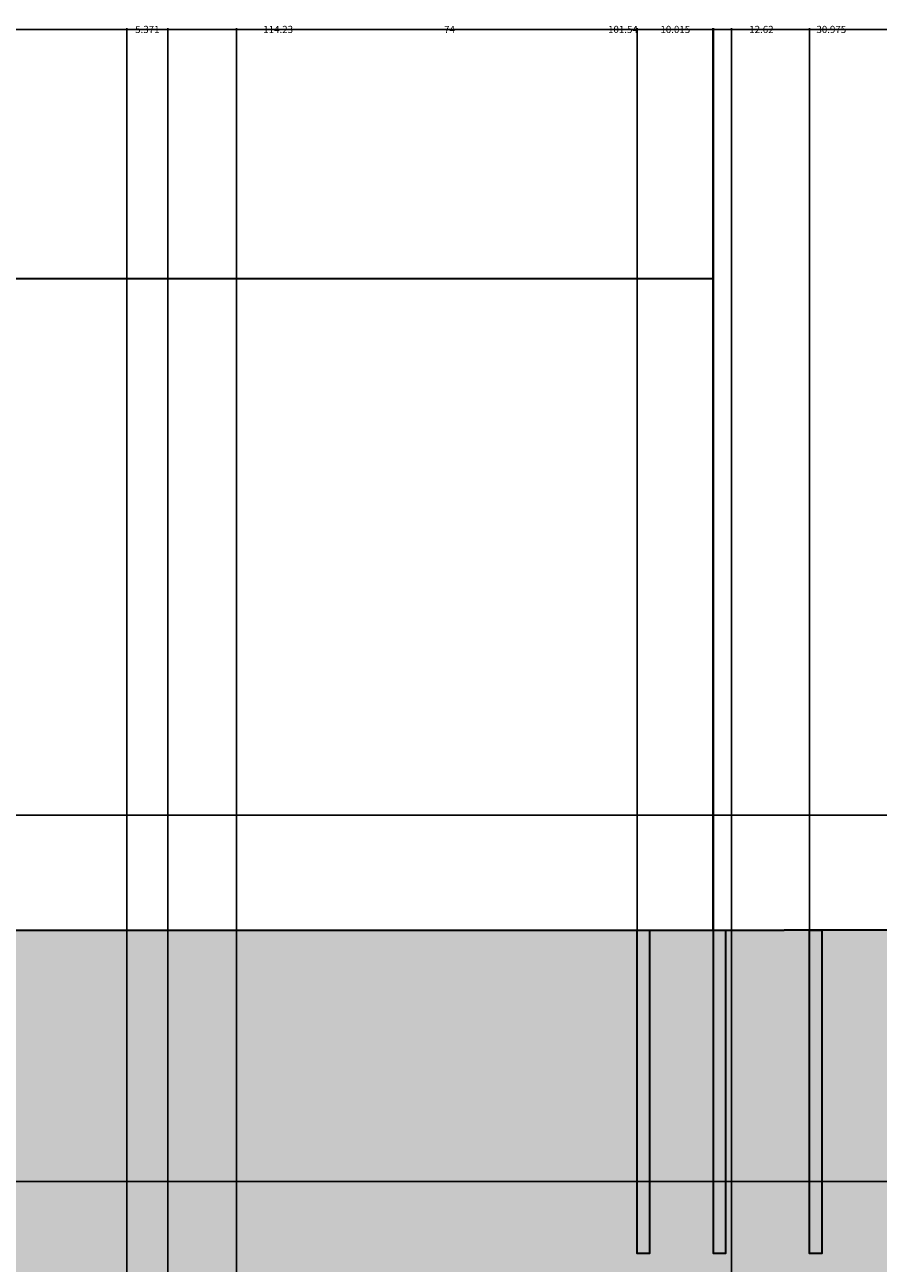
# Model space of a CAD drawing. Units: inches. Extents: x -5 to 714, y 84 to 644.
# Tile 10 of 20: x 108 to 220, y 481 to 644. Entities that reach past the tile are written whole.
import ezdxf

# ---------------------------------------------------------------- set-up
doc = ezdxf.new("R2010")
doc.units = ezdxf.units.IN
doc.header["$MEASUREMENT"] = 0
for name, color, linetype, lineweight in [('A-ANNO-DIMS', 2, 'Continuous', 18), ('A-ELEV', 7, 'Continuous', 35), ('A-ELEV-PATT', 8, 'Continuous', 13)]:
    doc.layers.add(name, color=color, linetype=linetype, lineweight=lineweight)
doc.styles.get("Standard").update_dxf_attribs({"font": 'arial.ttf'})
doc.dimstyles.get("Standard").update_dxf_attribs({"dimtxt": 0.9375, "dimasz": 0.18, "dimexe": 0.18, "dimexo": 0.0625, "dimgap": 0.09, "dimtad": 0, "dimtih": 1, "dimtoh": 1, "dimdec": 4, "dimzin": 0, "dimdsep": 46, "dimlunit": 4, "dimtxsty": 'Standard', "dimcen": 0.09, "dimadec": 0, "dimazin": 0, "dimtfac": 1, "dimtdec": 4, "dimtofl": 0, "dimtmove": 0, "dimatfit": 3, "dimfxl": 1, "dimtolj": 1, "dimtzin": 0, "dimarcsym": 0})

# ---------------------------------------------------------------- blocks, each defined once
blk = doc.blocks.new('*D10')
at = {"layer": 'A-ANNO-DIMS', "color": 0, "lineweight": -2, "transparency": 16777216}
for p, q in [((84.1, 610.79), (84.1, 643.61)), ((84.28, 643.43), (139.22, 643.43)), ((198.15, 643.43), (143.21, 643.43)), ((198.33, 610.79), (198.33, 643.61))]:
    blk.add_line(p, q, dxfattribs=at)
at = {"layer": 'A-ANNO-DIMS', "color": 0, "transparency": 16777216}
for points in [[(84.28, 643.46), (84.28, 643.4), (84.1, 643.43)], [(198.15, 643.46), (198.15, 643.4), (198.33, 643.43)]]:
    blk.add_solid(points, dxfattribs=at)
at = {"layer": 'Defpoints', "color": 0, "transparency": 16777216}
for p in [(198.33, 643.43), (84.1, 610.73), (198.33, 610.73)]:
    blk.add_point(p, dxfattribs=at)
at = {"layer": 'A-ANNO-DIMS', "color": 0, "transparency": 16777216, "insert": (141.22, 643.43), "char_height": 0.938, "attachment_point": 5}
blk.add_mtext('\\A1;114.23', dxfattribs=at)
blk = doc.blocks.new('*D11')
at = {"layer": 'A-ANNO-DIMS', "color": 0, "lineweight": -2, "transparency": 16777216}
for p, q in [((198.38, 525.26), (198.38, 643.61)), ((198.56, 643.43), (211.83, 643.43)), ((229.18, 643.43), (215.91, 643.43)), ((229.36, 525.26), (229.36, 643.61))]:
    blk.add_line(p, q, dxfattribs=at)
at = {"layer": 'A-ANNO-DIMS', "color": 0, "transparency": 16777216}
for points in [[(198.56, 643.46), (198.56, 643.4), (198.38, 643.43)], [(229.18, 643.46), (229.18, 643.4), (229.36, 643.43)]]:
    blk.add_solid(points, dxfattribs=at)
at = {"layer": 'Defpoints', "color": 0, "transparency": 16777216}
for p in [(229.36, 643.43), (198.38, 525.19), (229.36, 525.19)]:
    blk.add_point(p, dxfattribs=at)
at = {"layer": 'A-ANNO-DIMS', "color": 0, "transparency": 16777216, "insert": (213.87, 643.43), "char_height": 0.938, "attachment_point": 5}
blk.add_mtext('\\A1;30.975', dxfattribs=at)
blk = doc.blocks.new('*D16')
at = {"layer": 'A-ANNO-DIMS', "color": 0, "lineweight": -2, "transparency": 16777216}
for p, q in [((364.22, 540.29), (-2.74, 540.29)), ((-2.56, 540.11), (-2.56, 510.8)), ((-2.56, 480.35), (-2.56, 509.66)), ((364.22, 480.17), (-2.74, 480.17))]:
    blk.add_line(p, q, dxfattribs=at)
at = {"layer": 'A-ANNO-DIMS', "color": 0, "transparency": 16777216}
for points in [[(-2.59, 540.11), (-2.53, 540.11), (-2.56, 540.29)], [(-2.59, 480.35), (-2.53, 480.35), (-2.56, 480.17)]]:
    blk.add_solid(points, dxfattribs=at)
at = {"layer": 'Defpoints', "color": 0, "transparency": 16777216}
for p in [(-2.56, 540.29), (364.28, 540.29), (364.28, 480.17)]:
    blk.add_point(p, dxfattribs=at)
at = {"layer": 'A-ANNO-DIMS', "color": 0, "transparency": 16777216, "insert": (-2.56, 510.23), "char_height": 0.938, "attachment_point": 5}
blk.add_mtext('\\A1;60.11', dxfattribs=at)
blk = doc.blocks.new('*D17')
at = {"layer": 'A-ANNO-DIMS', "color": 0, "lineweight": -2, "transparency": 16777216}
for p, q in [((338.04, 525.19), (-2.74, 525.19)), ((-2.56, 525.01), (-2.56, 509.25)), ((-2.56, 492.35), (-2.56, 508.11)), ((338.04, 492.17), (-2.74, 492.17))]:
    blk.add_line(p, q, dxfattribs=at)
at = {"layer": 'A-ANNO-DIMS', "color": 0, "transparency": 16777216}
for points in [[(-2.59, 525.01), (-2.53, 525.01), (-2.56, 525.19)], [(-2.59, 492.35), (-2.53, 492.35), (-2.56, 492.17)]]:
    blk.add_solid(points, dxfattribs=at)
at = {"layer": 'Defpoints', "color": 0, "transparency": 16777216}
for p in [(-2.56, 525.19), (338.11, 525.19), (338.11, 492.17)]:
    blk.add_point(p, dxfattribs=at)
at = {"layer": 'A-ANNO-DIMS', "color": 0, "transparency": 16777216, "insert": (-2.56, 508.68), "char_height": 0.938, "attachment_point": 5}
blk.add_mtext('\\A1;33.03', dxfattribs=at)
blk = doc.blocks.new('*D21')
at = {"layer": 'A-ANNO-DIMS', "color": 0, "lineweight": -2, "transparency": 16777216}
for p, q in [((188.37, 482.78), (188.37, 643.61)), ((188.55, 643.43), (191.38, 643.43)), ((198.2, 643.43), (195.37, 643.43)), ((198.38, 482.78), (198.38, 643.61))]:
    blk.add_line(p, q, dxfattribs=at)
at = {"layer": 'A-ANNO-DIMS', "color": 0, "transparency": 16777216}
for points in [[(188.55, 643.46), (188.55, 643.4), (188.37, 643.43)], [(198.2, 643.46), (198.2, 643.4), (198.38, 643.43)]]:
    blk.add_solid(points, dxfattribs=at)
at = {"layer": 'Defpoints', "color": 0, "transparency": 16777216}
for p in [(198.38, 643.43), (188.37, 482.72), (198.38, 482.72)]:
    blk.add_point(p, dxfattribs=at)
at = {"layer": 'A-ANNO-DIMS', "color": 0, "transparency": 16777216, "insert": (193.38, 643.43), "char_height": 0.938, "attachment_point": 5}
blk.add_mtext('\\A1;10.015', dxfattribs=at)
blk = doc.blocks.new('*D22')
at = {"layer": 'A-ANNO-DIMS', "color": 0, "lineweight": -2, "transparency": 16777216}
for p, q in [((198.38, 482.78), (198.38, 643.61)), ((198.56, 643.43), (203.07, 643.43)), ((210.82, 643.43), (206.32, 643.43)), ((211, 482.78), (211, 643.61))]:
    blk.add_line(p, q, dxfattribs=at)
at = {"layer": 'A-ANNO-DIMS', "color": 0, "transparency": 16777216}
for points in [[(198.56, 643.46), (198.56, 643.4), (198.38, 643.43)], [(210.82, 643.46), (210.82, 643.4), (211, 643.43)]]:
    blk.add_solid(points, dxfattribs=at)
at = {"layer": 'Defpoints', "color": 0, "transparency": 16777216}
for p in [(211, 643.43), (198.38, 482.72), (211, 482.72)]:
    blk.add_point(p, dxfattribs=at)
at = {"layer": 'A-ANNO-DIMS', "color": 0, "transparency": 16777216, "insert": (204.69, 643.43), "char_height": 0.938, "attachment_point": 5}
blk.add_mtext('\\A1;12.62', dxfattribs=at)
blk = doc.blocks.new('*D23')
at = {"layer": 'A-ANNO-DIMS', "color": 0, "lineweight": -2, "transparency": 16777216}
for p, q in [((229.3, 525.19), (-2.74, 525.19)), ((-2.56, 525.01), (-2.56, 503.25)), ((-2.56, 480.35), (-2.56, 502.11)), ((229.3, 480.17), (-2.74, 480.17))]:
    blk.add_line(p, q, dxfattribs=at)
at = {"layer": 'A-ANNO-DIMS', "color": 0, "transparency": 16777216}
for points in [[(-2.59, 525.01), (-2.53, 525.01), (-2.56, 525.19)], [(-2.59, 480.35), (-2.53, 480.35), (-2.56, 480.17)]]:
    blk.add_solid(points, dxfattribs=at)
at = {"layer": 'Defpoints', "color": 0, "transparency": 16777216}
for p in [(-2.56, 525.19), (229.36, 525.19), (229.36, 480.17)]:
    blk.add_point(p, dxfattribs=at)
at = {"layer": 'A-ANNO-DIMS', "color": 0, "transparency": 16777216, "insert": (-2.56, 502.68), "char_height": 0.938, "attachment_point": 5}
blk.add_mtext('\\A1;45.02', dxfattribs=at)
blk = doc.blocks.new('*D24')
at = {"layer": 'A-ANNO-DIMS', "color": 0, "lineweight": -2, "transparency": 16777216}
for p, q in [((126.73, 480.23), (126.73, 643.61)), ((126.91, 643.43), (295.25, 643.43)), ((466.92, 643.43), (298.58, 643.43)), ((467.1, 480.23), (467.1, 643.61))]:
    blk.add_line(p, q, dxfattribs=at)
at = {"layer": 'A-ANNO-DIMS', "color": 0, "transparency": 16777216}
for points in [[(126.91, 643.46), (126.91, 643.4), (126.73, 643.43)], [(466.92, 643.46), (466.92, 643.4), (467.1, 643.43)]]:
    blk.add_solid(points, dxfattribs=at)
at = {"layer": 'Defpoints', "color": 0, "transparency": 16777216}
for p in [(467.1, 643.43), (126.73, 480.17), (467.1, 480.17)]:
    blk.add_point(p, dxfattribs=at)
at = {"layer": 'A-ANNO-DIMS', "color": 0, "transparency": 16777216, "insert": (296.91, 643.43), "char_height": 0.938, "attachment_point": 5}
blk.add_mtext('\\A1;340.4', dxfattribs=at)
blk = doc.blocks.new('*D31')
at = {"layer": 'A-ANNO-DIMS', "color": 0, "lineweight": -2, "transparency": 16777216}
for p, q in [((135.73, 345.26), (135.73, 643.61)), ((135.91, 643.43), (184.51, 643.43)), ((237.09, 643.43), (188.49, 643.43)), ((237.27, 345.26), (237.27, 643.61))]:
    blk.add_line(p, q, dxfattribs=at)
at = {"layer": 'A-ANNO-DIMS', "color": 0, "transparency": 16777216}
for points in [[(135.91, 643.46), (135.91, 643.4), (135.73, 643.43)], [(237.09, 643.46), (237.09, 643.4), (237.27, 643.43)]]:
    blk.add_solid(points, dxfattribs=at)
at = {"layer": 'Defpoints', "color": 0, "transparency": 16777216}
for p in [(237.27, 643.43), (135.73, 345.19), (237.27, 345.19)]:
    blk.add_point(p, dxfattribs=at)
at = {"layer": 'A-ANNO-DIMS', "color": 0, "transparency": 16777216, "insert": (186.5, 643.43), "char_height": 0.938, "attachment_point": 5}
blk.add_mtext('\\A1;101.54', dxfattribs=at)
blk = doc.blocks.new('*D47')
at = {"layer": 'A-ANNO-DIMS', "color": 0, "lineweight": -2, "transparency": 16777216}
for p, q in [((75.5, 336.27), (75.5, 643.61)), ((75.68, 643.43), (96.74, 643.43)), ((121.18, 643.43), (100.13, 643.43)), ((121.36, 336.27), (121.36, 643.61))]:
    blk.add_line(p, q, dxfattribs=at)
at = {"layer": 'A-ANNO-DIMS', "color": 0, "transparency": 16777216}
for points in [[(75.68, 643.46), (75.68, 643.4), (75.5, 643.43)], [(121.18, 643.46), (121.18, 643.4), (121.36, 643.43)]]:
    blk.add_solid(points, dxfattribs=at)
at = {"layer": 'Defpoints', "color": 0, "transparency": 16777216}
for p in [(121.36, 643.43), (75.5, 336.21), (121.36, 336.21)]:
    blk.add_point(p, dxfattribs=at)
at = {"layer": 'A-ANNO-DIMS', "color": 0, "transparency": 16777216, "insert": (98.43, 643.43), "char_height": 0.938, "attachment_point": 5}
blk.add_mtext('\\A1;45.85', dxfattribs=at)
blk = doc.blocks.new('*D48')
at = {"layer": 'A-ANNO-DIMS', "color": 0, "lineweight": -2, "transparency": 16777216}
for p, q in [((121.36, 336.27), (121.36, 643.61)), ((121.54, 643.43), (122.46, 643.43)), ((126.55, 643.43), (125.63, 643.43)), ((126.73, 345.26), (126.73, 643.61))]:
    blk.add_line(p, q, dxfattribs=at)
at = {"layer": 'A-ANNO-DIMS', "color": 0, "transparency": 16777216}
for points in [[(121.54, 643.46), (121.54, 643.4), (121.36, 643.43)], [(126.55, 643.46), (126.55, 643.4), (126.73, 643.43)]]:
    blk.add_solid(points, dxfattribs=at)
at = {"layer": 'Defpoints', "color": 0, "transparency": 16777216}
for p in [(126.73, 643.43), (126.73, 345.19), (121.36, 336.21)]:
    blk.add_point(p, dxfattribs=at)
at = {"layer": 'A-ANNO-DIMS', "color": 0, "transparency": 16777216, "insert": (124.04, 643.43), "char_height": 0.938, "attachment_point": 5}
blk.add_mtext('\\A1;5.371', dxfattribs=at)
blk = doc.blocks.new('*D49')
at = {"layer": 'A-ANNO-DIMS', "color": 0, "lineweight": -2, "transparency": 16777216}
for p, q in [((126.73, 302), (126.73, 643.61)), ((126.91, 643.43), (162.98, 643.43)), ((200.56, 643.43), (164.49, 643.43)), ((200.74, 302), (200.74, 643.61))]:
    blk.add_line(p, q, dxfattribs=at)
at = {"layer": 'A-ANNO-DIMS', "color": 0, "transparency": 16777216}
for points in [[(126.91, 643.46), (126.91, 643.4), (126.73, 643.43)], [(200.56, 643.46), (200.56, 643.4), (200.74, 643.43)]]:
    blk.add_solid(points, dxfattribs=at)
at = {"layer": 'Defpoints', "color": 0, "transparency": 16777216}
for p in [(200.74, 643.43), (126.73, 301.94), (200.74, 301.94)]:
    blk.add_point(p, dxfattribs=at)
at = {"layer": 'A-ANNO-DIMS', "color": 0, "transparency": 16777216, "insert": (163.73, 643.43), "char_height": 0.938, "attachment_point": 5}
blk.add_mtext('\\A1;74', dxfattribs=at)
blk = doc.blocks.new('*D51')
at = {"layer": 'A-ANNO-DIMS', "color": 0, "lineweight": -2, "transparency": 16777216}
for p, q in [((200.74, 201.26), (200.74, 643.61)), ((200.92, 643.43), (223.39, 643.43)), ((249.24, 643.43), (226.77, 643.43)), ((249.42, 201.26), (249.42, 643.61))]:
    blk.add_line(p, q, dxfattribs=at)
at = {"layer": 'A-ANNO-DIMS', "color": 0, "transparency": 16777216}
for points in [[(200.92, 643.46), (200.92, 643.4), (200.74, 643.43)], [(249.24, 643.46), (249.24, 643.4), (249.42, 643.43)]]:
    blk.add_solid(points, dxfattribs=at)
at = {"layer": 'Defpoints', "color": 0, "transparency": 16777216}
for p in [(249.42, 643.43), (200.74, 201.19), (249.42, 201.19)]:
    blk.add_point(p, dxfattribs=at)
at = {"layer": 'A-ANNO-DIMS', "color": 0, "transparency": 16777216, "insert": (225.08, 643.43), "char_height": 0.938, "attachment_point": 5}
blk.add_mtext('\\A1;48.68', dxfattribs=at)

msp = doc.modelspace()

# ---------------------------------------------------------------- hatches: boundary and pattern name
at = {"layer": 'A-ELEV-PATT', "transparency": 33554687}
h = msp.add_hatch(color=256, dxfattribs=at)
h.dxf.hatch_style = 1
h.paths.add_polyline_path([(188.3677, 525.1928), (67.9893, 525.1928), (67.9893, 489.1928), (67.9893, 345.1928), (126.7303, 345.1928), (126.7303, 480.1709), (229.3575, 480.1709), (229.3575, 525.1928), (212.6043, 525.1928), (212.6043, 482.7164), (211.0019, 482.7164), (211.0019, 525.1928), (207.6919, 525.1928), (199.9852, 525.1928), (199.9852, 482.7164), (198.3828, 482.7164), (198.3828, 525.1928), (189.9701, 525.1928), (189.9701, 482.7164), (188.3677, 482.7164)])
h.paths.add_polyline_path([(121.3589, 336.2066), (75.5048, 336.2066), (75.5048, 319.345), (121.3589, 319.345)])
h.paths.add_polyline_path([(121.3589, 319.345), (75.5048, 319.345), (75.5048, 302.3045), (121.3589, 302.3045)])
h.paths.add_polyline_path([(121.3589, 302.3045), (75.5048, 302.3045), (75.5048, 282.8561), (121.3589, 282.8561)])
h.paths.add_polyline_path([(121.3589, 282.8561), (75.5048, 282.8561), (75.5048, 261.5556), (121.3589, 261.5556)])
h.paths.add_polyline_path([(121.3589, 261.5556), (75.5048, 261.5556), (75.5048, 243.7009), (121.3589, 243.7009)])
h.paths.add_polyline_path([(121.3589, 243.7009), (75.5048, 243.7009), (75.5048, 223.5117), (121.3589, 223.5117)])
h.paths.add_polyline_path([(121.3589, 223.5117), (75.5048, 223.5117), (75.5048, 212.5836), (121.3589, 212.5836)])
h.paths.add_polyline_path([(121.3589, 212.5836), (75.5048, 212.5836), (75.5048, 201.1928), (121.3589, 201.1928)])
h.paths.add_polyline_path([(179.9335, 201.1928), (30.1395, 201.1928), (30.1395, 198.7054), (179.9335, 198.7054)])
h.paths.add_polyline_path([(187.6349, 201.1928), (179.9335, 201.1928), (179.9335, 198.7054), (179.9335, 141.1928), (269.2446, 141.1928), (269.2446, 201.1928), (263.4349, 201.1928), (263.4349, 152.1176), (187.6349, 152.1176)])
h.paths.add_polyline_path([(269.2446, 277.0513), (269.2446, 287.501), (269.2446, 306.6286), (578.0915, 306.6286), (578.0915, 201.1928), (593.428, 201.1928), (593.428, 315.0968), (584.4202, 315.0968), (259.0665, 315.0968), (259.0665, 201.1928), (263.4349, 201.1928), (269.2446, 201.1928)])
h = msp.add_hatch(color=256, dxfattribs=at)
h.dxf.hatch_style = 1
h.paths.add_polyline_path([(189.9701, 525.1928), (188.3677, 525.1928), (188.3677, 482.7164), (189.9701, 482.7164)])
h.paths.add_polyline_path([(199.9852, 525.1928), (198.3828, 525.1928), (198.3828, 482.7164), (199.9852, 482.7164)])
h.paths.add_polyline_path([(212.6043, 525.1928), (211.0019, 525.1928), (211.0019, 482.7164), (212.6043, 482.7164)])

# ---------------------------------------------------------------- linework, layer by layer
at = {"layer": 'A-ELEV'}
for p, q in [((79.1019, 610.7276), (198.3291, 610.7276)), ((198.3291, 610.7276), (198.3291, 525.1928)), ((67.9893, 525.1928), (207.6919, 525.1928)), ((229.3575, 525.1928), (207.6919, 525.1928))]:
    msp.add_line(p, q, dxfattribs=at)
for points in [[(188.3677, 525.1928), (189.9701, 525.1928), (189.9701, 482.7164), (188.3677, 482.7164)], [(198.3828, 525.1928), (199.9852, 525.1928), (199.9852, 482.7164), (198.3828, 482.7164)], [(211.0019, 525.1928), (212.6043, 525.1928), (212.6043, 482.7164), (211.0019, 482.7164)]]:
    msp.add_lwpolyline(points, close=True, dxfattribs=at)

# ---------------------------------------------------------------- dimensions: what is measured, and where the dimension line sits
at = {"layer": 'A-ANNO-DIMS'}
for base, p1, p2, override, picture, middle in [((121.3589, 643.4276), (75.5048, 336.2066), (121.3589, 336.2066), {"dimdec": 2, "dimlfac": 1, "dimrnd": 0, "dimzin": 0, "dimdsep": 46, "dimlunit": 2}, '*D47', (98.4319, 643.4276)), ((198.3291, 643.4276), (84.1027, 610.7276), (198.3291, 610.7276), {"dimdec": 2, "dimlfac": 1, "dimrnd": 0, "dimzin": 0, "dimdsep": 46, "dimlunit": 2}, '*D10', (141.2159, 643.4276)), ((126.7303, 643.4276), (121.3589, 336.2066), (126.7303, 345.1928), {"dimdec": 3, "dimlfac": 1, "dimrnd": 0, "dimzin": 0, "dimdsep": 46, "dimlunit": 2}, '*D48', (124.0446, 643.4276)), ((467.0994, 643.4276), (126.7303, 480.1709), (467.0994, 480.1709), {"dimdec": 1, "dimlfac": 1, "dimrnd": 0, "dimzin": 0, "dimdsep": 46, "dimlunit": 2}, '*D24', (296.9148, 643.4276)), ((200.7361, 643.4276), (126.7303, 301.9374), (200.7361, 301.9374), {"dimdec": 0, "dimlfac": 1, "dimrnd": 0, "dimzin": 0, "dimdsep": 46, "dimlunit": 2}, '*D49', (163.7332, 643.4276)), ((237.2654, 643.4276), (135.7303, 345.1928), (237.2654, 345.1928), {"dimdec": 2, "dimlfac": 1, "dimrnd": 0, "dimzin": 0, "dimdsep": 46, "dimlunit": 2}, '*D31', (186.4978, 643.4276)), ((198.3828, 643.4276), (188.3677, 482.7164), (198.3828, 482.7164), {"dimdec": 3, "dimlfac": 1, "dimrnd": 0, "dimzin": 0, "dimdsep": 46, "dimlunit": 2}, '*D21', (193.3752, 643.4276)), ((229.3575, 643.4276), (198.3828, 525.1928), (229.3575, 525.1928), {"dimdec": 3, "dimlfac": 1, "dimrnd": 0, "dimzin": 0, "dimdsep": 46, "dimlunit": 2}, '*D11', (213.8702, 643.4276)), ((211.0019, 643.4276), (198.3828, 482.7164), (211.0019, 482.7164), {"dimdec": 2, "dimlfac": 1, "dimrnd": 0, "dimzin": 0, "dimdsep": 46, "dimlunit": 2}, '*D22', (204.6923, 643.4276)), ((249.4181, 643.4276), (200.7361, 201.1928), (249.4181, 201.1928), {"dimdec": 2, "dimlfac": 1, "dimrnd": 0, "dimzin": 0, "dimdsep": 46, "dimlunit": 2}, '*D51', (225.0771, 643.4276))]:
    dim = msp.add_linear_dim(base=base, p1=p1, p2=p2, dimstyle='Standard', override=override, dxfattribs=at)
    dim.commit()
    dim.dimension.update_dxf_attribs({"geometry": picture, "text_midpoint": middle})
for base, p1, p2, picture, middle in [((-2.5605, 540.2857), (364.2809, 480.1709), (364.2809, 540.2857), '*D16', (-2.5605, 510.2283)), ((-2.5605, 525.1928), (338.106, 492.1651), (338.106, 525.1928), '*D17', (-2.5605, 508.679)), ((-2.5605, 525.1928), (229.3575, 480.1709), (229.3575, 525.1928), '*D23', (-2.5605, 502.6819))]:
    dim = msp.add_linear_dim(base=base, p1=p1, p2=p2, angle=90, dimstyle='Standard', override={"dimdec": 2, "dimlfac": 1, "dimrnd": 0, "dimzin": 0, "dimdsep": 46, "dimlunit": 2}, dxfattribs=at)
    dim.commit()
    dim.dimension.update_dxf_attribs({"geometry": picture, "text_midpoint": middle})

doc.saveas('drawing.dxf')
